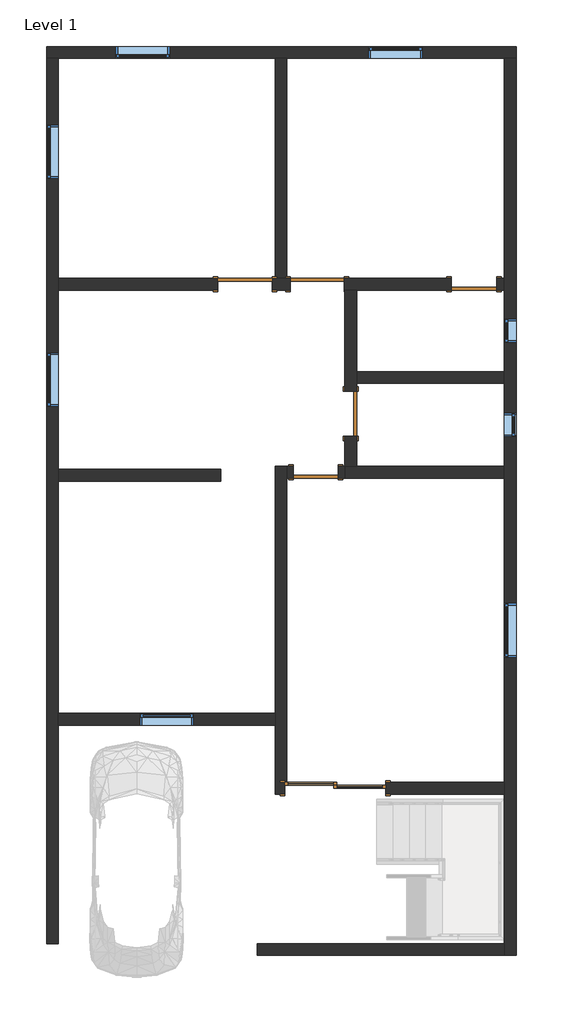
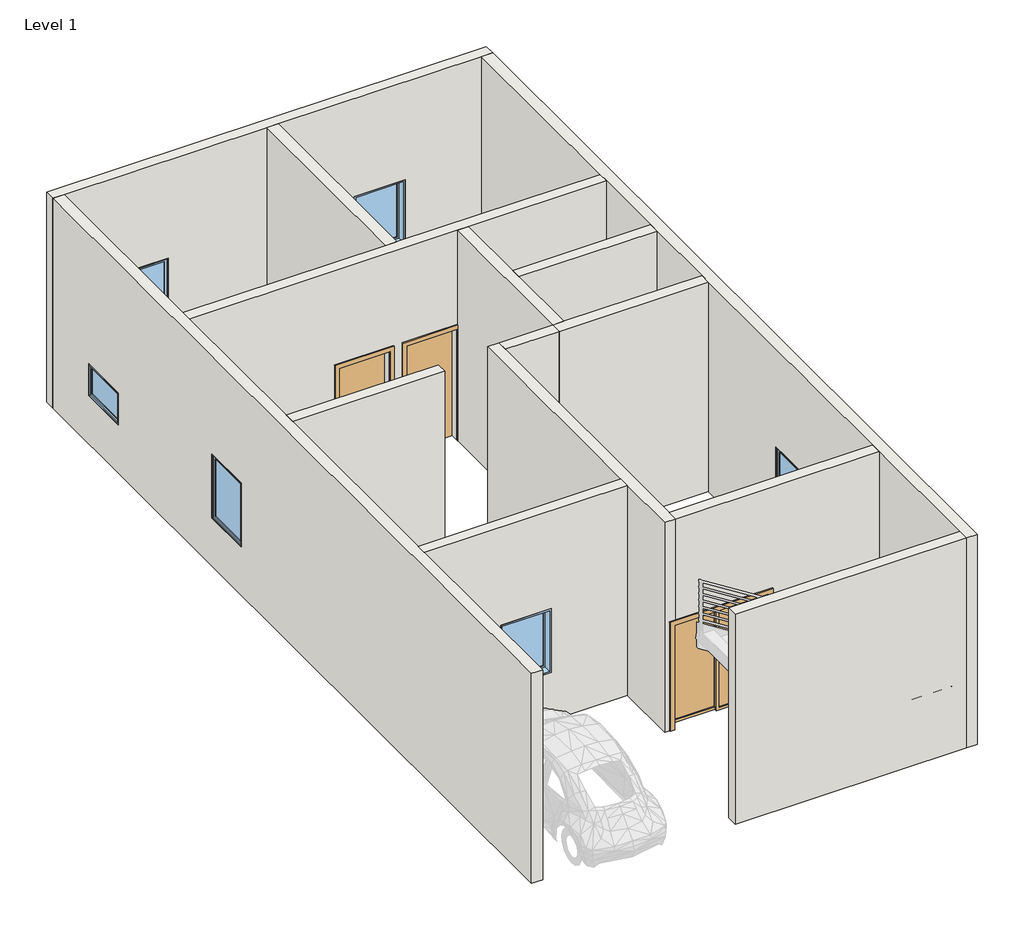
# One storey, part 1 of 4: 14 walls, 8 windows, 6 doors.
"""IFC4 building model written with IfcOpenShell, lengths in millimetres."""

from ifc_helpers import new_model, si_unit, frame, origin, origin_with_axes, place, context, project, spatial, polyline, outline, extrude, faceted_brep, transform, mapped, element, save
from components import m_door_double_sliding_1700_x_2000mm_9ea34811, m_single_flush_0762_x_2032mm_7341a4fb, m_single_flush_0762_x_2032mm_0c256fab, m_single_flush_0915_x_2134mm_6a9e8738, m_single_flush_0915_x_2134mm_727434cd, m_fixed_0406_x_0610mm_8205b201, m_fixed_0915_x_0610mm_70a843a6, m_fixed_0915_x_1220mm_488fb2fb

model = new_model("IFC4")

# Units and contexts
model_context = context("Model", 3, world=origin())
ifc_project = project(units=[si_unit("LENGTHUNIT", "METRE", prefix="MILLI")], contexts=[model_context])

# Site, building, storey
site = spatial("IfcSite", under=ifc_project)
building = spatial("IfcBuilding", under=site)
storey = spatial("IfcBuildingStorey", under=building, Name="Level 1", Elevation=0.0)

# Doors
placement = place(None, origin())
m_door_double_sliding_1700_x_2000mm_shape = m_door_double_sliding_1700_x_2000mm_9ea34811(model_context)
element("IfcDoor", 1, ObjectType="M_Door-Double-Sliding : 1700 x 2000mm", at=placement, inside=storey, context=model_context, shape_type="MappedRepresentation", body=[
    mapped(m_door_double_sliding_1700_x_2000mm_shape, transform((-4496.7496658, -1436.1048847, 0.0), x_axis=(1.0, 0.0, 0.0), y_axis=(0.0, 1.0, 0.0), z_axis=(0.0, 0.0, 1.0))),
])
m_single_flush_0762_x_2032mm_shape = m_single_flush_0762_x_2032mm_7341a4fb(model_context)
element("IfcDoor", 2, ObjectType="M_Single-Flush : 0762 x 2032mm", at=placement, inside=storey, context=model_context, shape_type="MappedRepresentation", body=[
    mapped(m_single_flush_0762_x_2032mm_shape, transform((-2153.5496658, 7201.4951153, 0.0), x_axis=(1.0, 0.0, 0.0), y_axis=(0.0, 1.0, 0.0), z_axis=(0.0, 0.0, 1.0))),
])
element("IfcDoor", 3, ObjectType="M_Single-Flush : 0762 x 2032mm", at=placement, inside=storey, context=model_context, shape_type="MappedRepresentation", body=[
    mapped(m_single_flush_0762_x_2032mm_shape, transform((-4236.3496658, 5015.4951153, 0.0), x_axis=(0.0, 1.0, 0.0), y_axis=(-1.0, 0.0, 0.0), z_axis=(0.0, 0.0, 1.0))),
])
m_single_flush_0762_x_2032mm_2_shape = m_single_flush_0762_x_2032mm_0c256fab(model_context)
element("IfcDoor", 4, ObjectType="M_Single-Flush : 0762 x 2032mm", at=placement, inside=storey, context=model_context, shape_type="MappedRepresentation", body=[
    mapped(m_single_flush_0762_x_2032mm_2_shape, transform((-4823.7496658, 4024.8951153, 0.0), x_axis=(-1.0, 0.0, 0.0), y_axis=(0.0, -1.0, 0.0), z_axis=(0.0, 0.0, 1.0))),
])
m_single_flush_0915_x_2134mm_shape = m_single_flush_0915_x_2134mm_6a9e8738(model_context)
element("IfcDoor", 5, ObjectType="M_Single-Flush : 0915 x 2134mm", at=placement, inside=storey, context=model_context, shape_type="MappedRepresentation", body=[
    mapped(m_single_flush_0915_x_2134mm_shape, transform((-6020.7496658, 7201.4951153, 0.0), x_axis=(1.0, 0.0, 0.0), y_axis=(0.0, 1.0, 0.0), z_axis=(0.0, 0.0, 1.0))),
])
m_single_flush_0915_x_2134mm_2_shape = m_single_flush_0915_x_2134mm_727434cd(model_context)
element("IfcDoor", 6, ObjectType="M_Single-Flush : 0915 x 2134mm", at=placement, inside=storey, context=model_context, shape_type="MappedRepresentation", body=[
    mapped(m_single_flush_0915_x_2134mm_2_shape, transform((-4801.5496658, 7201.4951153, 0.0), x_axis=(-1.0, 0.0, 0.0), y_axis=(0.0, -1.0, 0.0), z_axis=(0.0, 0.0, 1.0))),
])

# Walls
element("IfcWall", 7, ObjectType="Generic - 200mm", at=placement, inside=storey, context=model_context, shape_type="Brep", body=[
    faceted_brep([(-9368.7496658, 11011.4951153, 0.0), (-9168.7496658, 11011.4951153, 0.0), (-5511.1496658, 11011.4951153, 0.0), (-5311.1496658, 11011.4951153, 0.0), (-1643.9496658, 11011.4951153, 0.0), (-1443.9496658, 11011.4951153, 0.0), (-1443.9496658, 11011.4951153, 4000.0), (-1643.9496658, 11011.4951153, 4000.0), (-5311.1496658, 11011.4951153, 4000.0), (-5511.1496658, 11011.4951153, 4000.0), (-9168.7496658, 11011.4951153, 4000.0), (-9368.7496658, 11011.4951153, 4000.0), (-7287.2496658, 11011.4951153, 915.0), (-8202.2496658, 11011.4951153, 915.0), (-8202.2496658, 11011.4951153, 2135.0), (-7287.2496658, 11011.4951153, 2135.0), (-3935.0496658, 11011.4951153, 915.0), (-3935.0496658, 11011.4951153, 2135.0), (-3020.0496658, 11011.4951153, 2135.0), (-3020.0496658, 11011.4951153, 915.0), (-9368.7496658, 11211.4951153, 0.0), (-9368.7496658, 11211.4951153, 4000.0), (-1443.9496658, 11211.4951153, 4000.0), (-1443.9496658, 11211.4951153, 0.0), (-7287.2496658, 11211.4951153, 915.0), (-7287.2496658, 11211.4951153, 2135.0), (-8202.2496658, 11211.4951153, 2135.0), (-8202.2496658, 11211.4951153, 915.0), (-3935.0496658, 11211.4951153, 915.0), (-3020.0496658, 11211.4951153, 915.0), (-3020.0496658, 11211.4951153, 2135.0), (-3935.0496658, 11211.4951153, 2135.0)], [[[0, 1, 2, 3, 4, 5, 6, 7, 8, 9, 10, 11], [12, 13, 14, 15], [16, 17, 18, 19]], [[20, 21, 22, 23], [24, 25, 26, 27], [28, 29, 30, 31]], [[5, 4, 3, 2, 1, 0, 20, 23]], [[11, 10, 9, 8, 7, 6, 22, 21]], [[6, 5, 23, 22]], [[0, 11, 21, 20]], [[25, 24, 12, 15]], [[26, 25, 15, 14]], [[27, 26, 14, 13]], [[24, 27, 13, 12]], [[17, 16, 28, 31]], [[18, 17, 31, 30]], [[19, 18, 30, 29]], [[16, 19, 29, 28]]]),
])
element("IfcWall", 8, ObjectType="Generic - 200mm", at=placement, inside=storey, context=model_context, shape_type="Brep", body=[
    faceted_brep([(-1643.9496658, 11011.4951153, 0.0), (-1643.9496658, 7301.4951153, 0.0), (-1643.9496658, 7101.4951153, 0.0), (-1643.9496658, 5725.0951153, 0.0), (-1643.9496658, 5525.0951153, 0.0), (-1643.9496658, 4124.8951153, 0.0), (-1643.9496658, 3924.8951153, 0.0), (-1643.9496658, -1209.1048847, 0.0), (-1643.9496658, -1409.1048847, 0.0), (-1643.9496658, -3928.5048847, 0.0), (-1643.9496658, -4128.5048847, 0.0), (-1643.9496658, -4128.5048847, 4000.0), (-1643.9496658, -3928.5048847, 4000.0), (-1643.9496658, -1409.1048847, 4000.0), (-1643.9496658, -1209.1048847, 4000.0), (-1643.9496658, 3924.8951153, 4000.0), (-1643.9496658, 4124.8951153, 4000.0), (-1643.9496658, 5525.0951153, 4000.0), (-1643.9496658, 5725.0951153, 4000.0), (-1643.9496658, 7101.4951153, 4000.0), (-1643.9496658, 7301.4951153, 4000.0), (-1643.9496658, 11011.4951153, 4000.0), (-1643.9496658, 900.3951153, 915.0), (-1643.9496658, 1815.3951153, 915.0), (-1643.9496658, 1815.3951153, 2135.0), (-1643.9496658, 900.3951153, 2135.0), (-1643.9496658, 6210.2951153, 915.0), (-1643.9496658, 6616.2951153, 915.0), (-1643.9496658, 6616.2951153, 1525.0), (-1643.9496658, 6210.2951153, 1525.0), (-1643.9496658, 5027.9951153, 915.0), (-1643.9496658, 5027.9951153, 1525.0), (-1643.9496658, 4621.9951153, 1525.0), (-1643.9496658, 4621.9951153, 915.0), (-1443.9496658, 11011.4951153, 0.0), (-1443.9496658, 11011.4951153, 4000.0), (-1443.9496658, -4128.5048847, 4000.0), (-1443.9496658, -4128.5048847, 0.0), (-1443.9496658, 900.3951153, 915.0), (-1443.9496658, 900.3951153, 2135.0), (-1443.9496658, 1815.3951153, 2135.0), (-1443.9496658, 1815.3951153, 915.0), (-1443.9496658, 6210.2951153, 915.0), (-1443.9496658, 6210.2951153, 1525.0), (-1443.9496658, 6616.2951153, 1525.0), (-1443.9496658, 6616.2951153, 915.0), (-1443.9496658, 5027.9951153, 915.0), (-1443.9496658, 4621.9951153, 915.0), (-1443.9496658, 4621.9951153, 1525.0), (-1443.9496658, 5027.9951153, 1525.0)], [[[0, 1, 2, 3, 4, 5, 6, 7, 8, 9, 10, 11, 12, 13, 14, 15, 16, 17, 18, 19, 20, 21], [22, 23, 24, 25], [26, 27, 28, 29], [30, 31, 32, 33]], [[34, 35, 36, 37], [38, 39, 40, 41], [42, 43, 44, 45], [46, 47, 48, 49]], [[10, 9, 8, 7, 6, 5, 4, 3, 2, 1, 0, 34, 37]], [[21, 20, 19, 18, 17, 16, 15, 14, 13, 12, 11, 36, 35]], [[0, 21, 35, 34]], [[39, 38, 22, 25]], [[40, 39, 25, 24]], [[41, 40, 24, 23]], [[38, 41, 23, 22]], [[43, 42, 26, 29]], [[44, 43, 29, 28]], [[45, 44, 28, 27]], [[42, 45, 27, 26]], [[31, 30, 46, 49]], [[32, 31, 49, 48]], [[33, 32, 48, 47]], [[30, 33, 47, 46]], [[11, 10, 37, 36]]]),
])
element("IfcWall", 9, ObjectType="Generic - 200mm", at=placement, inside=storey, context=model_context, shape_type="Brep", body=[
    faceted_brep([(-9168.7496658, -3928.5048847, 0.0), (-9168.7496658, -242.3048847, 0.0), (-9168.7496658, -42.3048847, 0.0), (-9168.7496658, 3877.2951153, 0.0), (-9168.7496658, 4077.2951153, 0.0), (-9168.7496658, 7101.4951153, 0.0), (-9168.7496658, 7301.4951153, 0.0), (-9168.7496658, 11011.4951153, 0.0), (-9168.7496658, 11011.4951153, 4000.0), (-9168.7496658, 7301.4951153, 4000.0), (-9168.7496658, 7101.4951153, 4000.0), (-9168.7496658, 4077.2951153, 4000.0), (-9168.7496658, 3877.2951153, 4000.0), (-9168.7496658, -42.3048847, 4000.0), (-9168.7496658, -242.3048847, 4000.0), (-9168.7496658, -3928.5048847, 4000.0), (-9168.7496658, 5131.8951153, 915.0), (-9168.7496658, 5131.8951153, 2135.0), (-9168.7496658, 6046.8951153, 2135.0), (-9168.7496658, 6046.8951153, 915.0), (-9168.7496658, 8977.5951153, 915.0), (-9168.7496658, 8977.5951153, 1525.0), (-9168.7496658, 9892.5951153, 1525.0), (-9168.7496658, 9892.5951153, 915.0), (-9368.7496658, -3928.5048847, 0.0), (-9368.7496658, -3928.5048847, 4000.0), (-9368.7496658, 11011.4951153, 4000.0), (-9368.7496658, 11011.4951153, 0.0), (-9368.7496658, 5131.8951153, 915.0), (-9368.7496658, 6046.8951153, 915.0), (-9368.7496658, 6046.8951153, 2135.0), (-9368.7496658, 5131.8951153, 2135.0), (-9368.7496658, 8977.5951153, 915.0), (-9368.7496658, 9892.5951153, 915.0), (-9368.7496658, 9892.5951153, 1525.0), (-9368.7496658, 8977.5951153, 1525.0)], [[[0, 1, 2, 3, 4, 5, 6, 7, 8, 9, 10, 11, 12, 13, 14, 15], [16, 17, 18, 19], [20, 21, 22, 23]], [[24, 25, 26, 27], [28, 29, 30, 31], [32, 33, 34, 35]], [[7, 6, 5, 4, 3, 2, 1, 0, 24, 27]], [[15, 14, 13, 12, 11, 10, 9, 8, 26, 25]], [[0, 15, 25, 24]], [[8, 7, 27, 26]], [[17, 16, 28, 31]], [[18, 17, 31, 30]], [[19, 18, 30, 29]], [[16, 19, 29, 28]], [[21, 20, 32, 35]], [[22, 21, 35, 34]], [[23, 22, 34, 33]], [[20, 23, 33, 32]]]),
])
element("IfcWall", 10, ObjectType="Generic - 200mm", at=placement, inside=storey, context=model_context, shape_type="Brep", body=[
    faceted_brep([(-1772.5496658, 7101.4951153, 2032.0), (-1772.5496658, 7101.4951153, 0.0), (-1643.9496658, 7101.4951153, 0.0), (-1643.9496658, 7101.4951153, 4000.0), (-4136.3496658, 7101.4951153, 4000.0), (-4336.3496658, 7101.4951153, 4000.0), (-9168.7496658, 7101.4951153, 4000.0), (-9168.7496658, 7101.4951153, 0.0), (-6478.2496658, 7101.4951153, 0.0), (-6478.2496658, 7101.4951153, 2134.0), (-5563.2496658, 7101.4951153, 2134.0), (-5563.2496658, 7101.4951153, 0.0), (-5259.0496658, 7101.4951153, 0.0), (-5259.0496658, 7101.4951153, 2134.0), (-4344.0496658, 7101.4951153, 2134.0), (-4344.0496658, 7101.4951153, 0.0), (-4336.3496658, 7101.4951153, 0.0), (-4136.3496658, 7101.4951153, 0.0), (-2534.5496658, 7101.4951153, 0.0), (-2534.5496658, 7101.4951153, 2032.0), (-1643.9496658, 7301.4951153, 0.0), (-1772.5496658, 7301.4951153, 0.0), (-1772.5496658, 7301.4951153, 2032.0), (-2534.5496658, 7301.4951153, 2032.0), (-2534.5496658, 7301.4951153, 0.0), (-4344.0496658, 7301.4951153, 0.0), (-4344.0496658, 7301.4951153, 2134.0), (-5259.0496658, 7301.4951153, 2134.0), (-5259.0496658, 7301.4951153, 0.0), (-5311.1496658, 7301.4951153, 0.0), (-5511.1496658, 7301.4951153, 0.0), (-5563.2496658, 7301.4951153, 0.0), (-5563.2496658, 7301.4951153, 2134.0), (-6478.2496658, 7301.4951153, 2134.0), (-6478.2496658, 7301.4951153, 0.0), (-9168.7496658, 7301.4951153, 0.0), (-9168.7496658, 7301.4951153, 4000.0), (-5511.1496658, 7301.4951153, 4000.0), (-5311.1496658, 7301.4951153, 4000.0), (-1643.9496658, 7301.4951153, 4000.0)], [[[0, 1, 2, 3, 4, 5, 6, 7, 8, 9, 10, 11, 12, 13, 14, 15, 16, 17, 18, 19]], [[20, 21, 22, 23, 24, 25, 26, 27, 28, 29, 30, 31, 32, 33, 34, 35, 36, 37, 38, 39]], [[8, 7, 35, 34]], [[31, 30, 29, 28, 12, 11]], [[2, 1, 21, 20]], [[18, 17, 16, 15, 25, 24]], [[6, 5, 4, 3, 39, 38, 37, 36]], [[7, 6, 36, 35]], [[3, 2, 20, 39]], [[32, 31, 11, 10]], [[33, 32, 10, 9]], [[34, 33, 9, 8]], [[13, 12, 28, 27]], [[14, 13, 27, 26]], [[15, 14, 26, 25]], [[22, 21, 1, 0]], [[23, 22, 0, 19]], [[24, 23, 19, 18]]]),
])
element("IfcWall", 11, ObjectType="Generic - 200mm", at=placement, inside=storey, context=model_context, shape_type="SweptSolid", body=[
    extrude(outline(polyline([(-5311.1496658, 11011.4951153), (-5311.1496658, 7301.4951153), (-5511.1496658, 7301.4951153), (-5511.1496658, 11011.4951153), (-5311.1496658, 11011.4951153)])), origin_with_axes(), (0.0, 0.0, 1.0), 4000.0),
])
element("IfcWall", 12, ObjectType="Generic - 200mm", at=placement, inside=storey, context=model_context, shape_type="SweptSolid", body=[
    extrude(outline(polyline([(-4136.3496658, 5725.0951153), (-1643.9496658, 5725.0951153), (-1643.9496658, 5525.0951153), (-4136.3496658, 5525.0951153), (-4136.3496658, 5725.0951153)])), origin_with_axes(), (0.0, 0.0, 1.0), 4000.0),
])
element("IfcWall", 13, ObjectType="Generic - 200mm", at=placement, inside=storey, context=model_context, shape_type="Brep", body=[
    faceted_brep([(-4136.3496658, 5396.4951153, 2032.0), (-4136.3496658, 5396.4951153, 0.0), (-4136.3496658, 5525.0951153, 0.0), (-4136.3496658, 5725.0951153, 0.0), (-4136.3496658, 7101.4951153, 0.0), (-4136.3496658, 7101.4951153, 4000.0), (-4136.3496658, 5725.0951153, 4000.0), (-4136.3496658, 5525.0951153, 4000.0), (-4136.3496658, 4124.8951153, 4000.0), (-4136.3496658, 4124.8951153, 0.0), (-4136.3496658, 4634.4951153, 0.0), (-4136.3496658, 4634.4951153, 2032.0), (-4336.3496658, 7101.4951153, 0.0), (-4336.3496658, 5396.4951153, 0.0), (-4336.3496658, 5396.4951153, 2032.0), (-4336.3496658, 4634.4951153, 2032.0), (-4336.3496658, 4634.4951153, 0.0), (-4336.3496658, 4124.8951153, 0.0), (-4336.3496658, 4124.8951153, 4000.0), (-4336.3496658, 7101.4951153, 4000.0)], [[[0, 1, 2, 3, 4, 5, 6, 7, 8, 9, 10, 11]], [[12, 13, 14, 15, 16, 17, 18, 19]], [[10, 9, 17, 16]], [[4, 3, 2, 1, 13, 12]], [[8, 7, 6, 5, 19, 18]], [[5, 4, 12, 19]], [[9, 8, 18, 17]], [[14, 13, 1, 0]], [[15, 14, 0, 11]], [[16, 15, 11, 10]]]),
])
element("IfcWall", 14, ObjectType="Generic - 200mm", at=placement, inside=storey, context=model_context, shape_type="Brep", body=[
    faceted_brep([(-1643.9496658, 4124.8951153, 0.0), (-4136.3496658, 4124.8951153, 0.0), (-4336.3496658, 4124.8951153, 0.0), (-4336.3496658, 4124.8951153, 4000.0), (-4136.3496658, 4124.8951153, 4000.0), (-1643.9496658, 4124.8951153, 4000.0), (-1643.9496658, 3924.8951153, 0.0), (-1643.9496658, 3924.8951153, 4000.0), (-4336.3496658, 3924.8951153, 4000.0), (-4336.3496658, 3924.8951153, 0.0)], [[[0, 1, 2, 3, 4, 5]], [[6, 7, 8, 9]], [[2, 1, 0, 6, 9]], [[5, 4, 3, 8, 7]], [[0, 5, 7, 6]], [[3, 2, 9, 8]]]),
])
element("IfcWall", 15, ObjectType="Generic - 200mm", at=placement, inside=storey, context=model_context, shape_type="SweptSolid", body=[
    extrude(outline(polyline([(-6425.5496658, 3877.2951153), (-9168.7496658, 3877.2951153), (-9168.7496658, 4077.2951153), (-6425.5496658, 4077.2951153), (-6425.5496658, 3877.2951153)])), origin_with_axes(), (0.0, 0.0, 1.0), 4000.0),
])
element("IfcWall", 16, ObjectType="Generic - 200mm", at=placement, inside=storey, context=model_context, shape_type="Brep", body=[
    faceted_brep([(-5511.1496658, 4124.8951153, 0.0), (-5511.1496658, -42.3048847, 0.0), (-5511.1496658, -242.3048847, 0.0), (-5511.1496658, -1409.1048847, 0.0), (-5511.1496658, -1409.1048847, 4000.0), (-5511.1496658, -242.3048847, 4000.0), (-5511.1496658, -42.3048847, 4000.0), (-5511.1496658, 4124.8951153, 4000.0), (-5311.1496658, 4124.8951153, 4000.0), (-5311.1496658, 3924.8951153, 4000.0), (-5311.1496658, -1209.1048847, 4000.0), (-5311.1496658, -1409.1048847, 4000.0), (-5311.1496658, -1409.1048847, 2000.0), (-5311.1496658, -1209.1048847, 2000.0), (-5311.1496658, -1209.1048847, 0.0), (-5311.1496658, 3924.8951153, 0.0), (-5311.1496658, 4124.8951153, 0.0), (-5346.7496658, -1209.1048847, 0.0), (-5346.7496658, -1409.1048847, 0.0), (-5346.7496658, -1409.1048847, 2000.0), (-5346.7496658, -1209.1048847, 2000.0)], [[[0, 1, 2, 3, 4, 5, 6, 7]], [[8, 9, 10, 11, 12, 13, 14, 15, 16]], [[3, 2, 1, 0, 16, 15, 14, 17, 18]], [[7, 6, 5, 4, 11, 10, 9, 8]], [[4, 3, 18, 19, 12, 11]], [[0, 7, 8, 16]], [[20, 17, 14, 13]], [[17, 20, 19, 18]], [[19, 20, 13, 12]]]),
])
element("IfcWall", 17, ObjectType="Generic - 200mm", at=placement, inside=storey, context=model_context, shape_type="SweptSolid", body=[
    extrude(outline(polyline([(4000.0, -1643.9496658), (4000.0, -5311.1496658), (2000.0, -5311.1496658), (2000.0, -3646.7496658), (0.0, -3646.7496658), (0.0, -1643.9496658), (4000.0, -1643.9496658)])), frame((0.0, -1409.1048847, 0.0), z_axis=(0.0, 1.0, 0.0), x_axis=(0.0, 0.0, 1.0)), (0.0, 0.0, 1.0), 200.0),
])
element("IfcWall", 18, ObjectType="Generic - 200mm", at=placement, inside=storey, context=model_context, shape_type="SweptSolid", body=[
    extrude(outline(polyline([(0.0, -5511.1496658), (4000.0, -5511.1496658), (4000.0, -9168.7496658), (0.0, -9168.7496658), (0.0, -5511.1496658)]), holes=[polyline([(915.0, -7797.4496658), (2135.0, -7797.4496658), (2135.0, -6882.4496658), (915.0, -6882.4496658), (915.0, -7797.4496658)])]), frame((0.0, -242.3048847, 0.0), z_axis=(0.0, 1.0, 0.0), x_axis=(0.0, 0.0, 1.0)), (0.0, 0.0, 1.0), 200.0),
])
element("IfcWall", 19, ObjectType="Generic - 200mm", at=placement, inside=storey, context=model_context, shape_type="SweptSolid", body=[
    extrude(outline(polyline([(0.0, -5311.1496658), (0.0, -5204.7496658), (2032.0, -5204.7496658), (2032.0, -4442.7496658), (0.0, -4442.7496658), (0.0, -4336.3496658), (4000.0, -4336.3496658), (4000.0, -5311.1496658), (0.0, -5311.1496658)])), frame((0.0, 3924.8951153, 0.0), z_axis=(0.0, 1.0, 0.0), x_axis=(0.0, 0.0, 1.0)), (0.0, 0.0, 1.0), 200.0),
])
element("IfcWall", 20, ObjectType="Generic - 200mm", at=placement, inside=storey, context=model_context, shape_type="SweptSolid", body=[
    extrude(outline(polyline([(-5811.1496658, -3928.5048847), (-1643.9496658, -3928.5048847), (-1643.9496658, -4128.5048847), (-5811.1496658, -4128.5048847), (-5811.1496658, -3928.5048847)])), origin_with_axes(), (0.0, 0.0, 1.0), 4000.0),
])

# Windows
m_fixed_0406_x_0610mm_shape = m_fixed_0406_x_0610mm_8205b201(model_context)
element("IfcWindow", 21, ObjectType="M_Fixed : 0406 x 0610mm", at=placement, inside=storey, context=model_context, shape_type="MappedRepresentation", body=[
    mapped(m_fixed_0406_x_0610mm_shape, transform((-1530.9496658, 6413.2951153, 0.0), x_axis=(0.0, 1.0, 0.0), y_axis=(-1.0, 0.0, 0.0), z_axis=(0.0, 0.0, 1.0))),
])
element("IfcWindow", 22, ObjectType="M_Fixed : 0406 x 0610mm", at=placement, inside=storey, context=model_context, shape_type="MappedRepresentation", body=[
    mapped(m_fixed_0406_x_0610mm_shape, transform((-1556.9496658, 4824.9951153, 0.0), x_axis=(0.0, -1.0, 0.0), y_axis=(1.0, 0.0, 0.0), z_axis=(0.0, 0.0, 1.0))),
])
m_fixed_0915_x_0610mm_shape = m_fixed_0915_x_0610mm_70a843a6(model_context)
element("IfcWindow", 23, ObjectType="M_Fixed : 0915 x 0610mm", at=placement, inside=storey, context=model_context, shape_type="MappedRepresentation", body=[
    mapped(m_fixed_0915_x_0610mm_shape, transform((-9255.7496658, 9435.0951153, 0.0), x_axis=(0.0, 1.0, 0.0), y_axis=(-1.0, 0.0, 0.0), z_axis=(0.0, 0.0, 1.0))),
])
m_fixed_0915_x_1220mm_shape = m_fixed_0915_x_1220mm_488fb2fb(model_context)
element("IfcWindow", 24, ObjectType="M_Fixed : 0915 x 1220mm", at=placement, inside=storey, context=model_context, shape_type="MappedRepresentation", body=[
    mapped(m_fixed_0915_x_1220mm_shape, transform((-7744.7496658, 11124.4951153, 0.0), x_axis=(-1.0, 0.0, 0.0), y_axis=(0.0, -1.0, 0.0), z_axis=(0.0, 0.0, 1.0))),
])
element("IfcWindow", 25, ObjectType="M_Fixed : 0915 x 1220mm", at=placement, inside=storey, context=model_context, shape_type="MappedRepresentation", body=[
    mapped(m_fixed_0915_x_1220mm_shape, transform((-3477.5496658, 11098.4951153, 0.0), x_axis=(1.0, 0.0, 0.0), y_axis=(0.0, 1.0, 0.0), z_axis=(0.0, 0.0, 1.0))),
])
element("IfcWindow", 26, ObjectType="M_Fixed : 0915 x 1220mm", at=placement, inside=storey, context=model_context, shape_type="MappedRepresentation", body=[
    mapped(m_fixed_0915_x_1220mm_shape, transform((-9255.7496658, 5589.3951153, 0.0), x_axis=(0.0, 1.0, 0.0), y_axis=(-1.0, 0.0, 0.0), z_axis=(0.0, 0.0, 1.0))),
])
element("IfcWindow", 27, ObjectType="M_Fixed : 0915 x 1220mm", at=placement, inside=storey, context=model_context, shape_type="MappedRepresentation", body=[
    mapped(m_fixed_0915_x_1220mm_shape, transform((-7339.9496658, -155.3048847, 0.0), x_axis=(1.0, 0.0, 0.0), y_axis=(0.0, 1.0, 0.0), z_axis=(0.0, 0.0, 1.0))),
])
element("IfcWindow", 28, ObjectType="M_Fixed : 0915 x 1220mm", at=placement, inside=storey, context=model_context, shape_type="MappedRepresentation", body=[
    mapped(m_fixed_0915_x_1220mm_shape, transform((-1530.9496658, 1357.8951153, 0.0), x_axis=(0.0, 1.0, 0.0), y_axis=(-1.0, 0.0, 0.0), z_axis=(0.0, 0.0, 1.0))),
])

save(model, "model.ifc")

# Revit data of these elements
# Type "M_Door-Double-Sliding : 1700 x 2000mm"
#   Type Mark = "22"
#   Construction Type Id = "opn-d45"
#   Assembly Code = "C1020"
#   Analytic Construction = "Wood frame, double glass door "
#   Thickness = 0' - 1.9685"
#   Thermal Resistance (R) = 0.31964 (m²·K)/W
#   Heat Transfer Coefficient (U) = 3.12872 W/(m²·K)
#   Height = 6' - 6.74016"
#   Rail Width = 0' - 1.9685"
#   Stiles = 0' - 1.9685"
#   Trim Projection Ext = 0' - 0.98425"
#   Trim Projection Int = 0' - 0.98425"
#   Trim Width = 0' - 3.14961"
#   Width = 5' - 6.92913"
#   Define Thermal Properties by = 1
#   Glazing = Glass
#   Panel Material = Wood - Birch - Solid Stained Light Low Gloss
#   Trim Material = Paint - Sienna
#   Visual Light Transmittance = 0
#   Solar Heat Gain Coefficient = 0
#   Function = (empty or 0)
#   Wall Closure = (empty or 0)
# Type "M_Single-Flush : 0762 x 2032mm"
#   Type Mark = "19"
#   Thickness = 0' - 2.00787"
#   Height = 6' - 8"
#   Trim Projection Ext = 0' - 0.98425"
#   Trim Projection Int = 0' - 0.98425"
#   Trim Width = 0' - 2.99213"
#   Width = 2' - 6"
#   Door Material = Door - Panel
#   Frame Material = Door - Frame
#   Function = (empty or 0)
#   Wall Closure = (empty or 0)
# Type "M_Single-Flush : 0915 x 2134mm"
#   Type Mark = "15"
#   Thickness = 0' - 2.00787"
#   Height = 7' - 0.01575"
#   Trim Projection Ext = 0' - 0.98425"
#   Trim Projection Int = 0' - 0.98425"
#   Trim Width = 0' - 2.99213"
#   Width = 3' - 0.02362"
#   Door Material = Door - Panel
#   Frame Material = Door - Frame
#   Function = (empty or 0)
#   Wall Closure = (empty or 0)
# Type "Generic - 200mm"
#   Layers, outside or top first: 0' - 7.87402" no material (function 1)
# Type "M_Fixed : 0406 x 0610mm"
#   Type Mark = "10"
#   Height = 2' - 0.01575"
#   Default Sill Height = 3' - 0.02362"
#   Width = 1' - 3.98425"
#   Window Inset = 0' - 0.74803"
#   Frame Exterior Material = Sash
#   Frame Interior Material = Sash
#   Glass Pane Material = Glass
#   Sash = Sash
#   Wall Closure = (empty or 0)
# Type "M_Fixed : 0915 x 0610mm"
#   Type Mark = "14"
#   Height = 2' - 0.01575"
#   Default Sill Height = 3' - 0.02362"
#   Width = 3' - 0.02362"
#   Window Inset = 0' - 0.74803"
#   Frame Exterior Material = Sash
#   Frame Interior Material = Sash
#   Glass Pane Material = Glass
#   Sash = Sash
#   Wall Closure = (empty or 0)
# Type "M_Fixed : 0915 x 1220mm"
#   Type Mark = "15"
#   Height = 4' - 0.0315"
#   Default Sill Height = 3' - 0.02362"
#   Width = 3' - 0.02362"
#   Window Inset = 0' - 0.74803"
#   Frame Exterior Material = Sash
#   Frame Interior Material = Sash
#   Glass Pane Material = Glass
#   Sash = Sash
#   Wall Closure = (empty or 0)
# Element 1 (IfcDoor, "M_Door-Double-Sliding : 1700 x 2000mm")
#   Phase Created = New Construction
#   Materials on its faces: "Paint - Sienna", "Wood - Birch - Solid Stained Light Low Gloss", "Glass"
# Elements 2, 3, 4 (IfcDoor, "M_Single-Flush : 0762 x 2032mm")
#   Phase Created = New Construction
#   Materials on its faces: "Door - Frame", "Door - Panel"
# Elements 5, 6 (IfcDoor, "M_Single-Flush : 0915 x 2134mm")
#   Phase Created = New Construction
#   Materials on its faces: "Door - Frame", "Door - Panel"
# Elements 7, 8, 9, 10, 11, 12, 13, 14, 15, 16, 17, 18, 19, 20 (IfcWall, "Generic - 200mm")
#   Top Offset = 0' - 0"
#   Base Offset = 0' - 0"
#   wall height = 13' - 1.48031"
#   Phase Created = New Construction
#   Base Constraint = Level 1
#   Top Constraint = Level 2
#   Materials on its faces: "Default Wall"
# Element 21 (IfcWindow, "M_Fixed : 0406 x 0610mm")
#   Mark = "11"
#   Phase Created = New Construction
#   Materials on its faces: "Sash", "Glass"
# Element 22 (IfcWindow, "M_Fixed : 0406 x 0610mm")
#   Mark = "12"
#   Phase Created = New Construction
#   Materials on its faces: "Sash", "Glass"
# Element 23 (IfcWindow, "M_Fixed : 0915 x 0610mm")
#   Mark = "13"
#   Phase Created = New Construction
#   Materials on its faces: "Sash", "Glass"
# Element 24 (IfcWindow, "M_Fixed : 0915 x 1220mm")
#   Mark = "6"
#   Phase Created = New Construction
#   Materials on its faces: "Sash", "Glass"
# Element 25 (IfcWindow, "M_Fixed : 0915 x 1220mm")
#   Mark = "7"
#   Phase Created = New Construction
#   Materials on its faces: "Sash", "Glass"
# Element 26 (IfcWindow, "M_Fixed : 0915 x 1220mm")
#   Mark = "8"
#   Phase Created = New Construction
#   Materials on its faces: "Sash", "Glass"
# Element 27 (IfcWindow, "M_Fixed : 0915 x 1220mm")
#   Mark = "9"
#   Phase Created = New Construction
#   Materials on its faces: "Sash", "Glass"
# Element 28 (IfcWindow, "M_Fixed : 0915 x 1220mm")
#   Mark = "10"
#   Phase Created = New Construction
#   Materials on its faces: "Sash", "Glass"
# Materials
#   "Glass": class "Glass", colour RGB 218 227 224, transparency 0.85, Description = "Soda Lime Glass", Cost = 0
#   "Wood - Birch - Solid Stained Light Low Gloss": class "Wood", colour RGB 210 159 95, transparency 0, Cost = 0
#   "Paint - Sienna": colour RGB 118 70 51, transparency 0, Cost = 0
#   "Door - Panel": class "Wood", colour RGB 114 82 51, transparency 0
#   "Door - Frame": colour RGB 153 76 43, transparency 0
#   "Sash": class "Wood", colour RGB 136 99 55, transparency 0
#   "Default Wall": colour RGB 80 80 80, transparency 0
